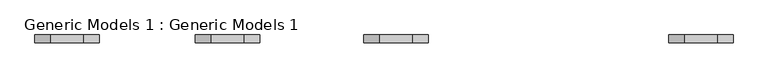
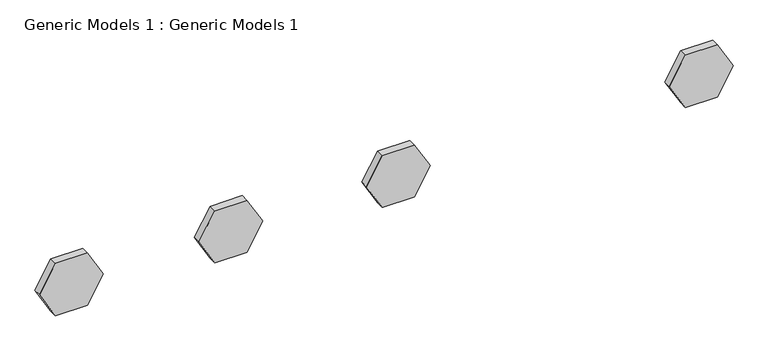
"""IFC4 building model written with IfcOpenShell, lengths in millimetres: proxy geometry, Generic Models 1 : Generic Models 1."""

from ifc_helpers import new_model, si_unit, frame, origin, place, context, project, spatial, polyline, outline, extrude, source, transform, mapped, element, save


def generic_models_1_generic_models_1_46fdab30(model_context):
    return source(origin(), model_context, "Body", "SweptSolid", [
        extrude(outline(polyline([(1354.8156911, 5498.4896844), (1354.8156911, 4888.8896844), (826.8866049, 4584.0896844), (298.9575188, 4888.8896844), (298.9575188, 5498.4896844), (826.8866049, 5803.2896844), (1354.8156911, 5498.4896844)])), frame((0.0, -9884.41366, 0.0), z_axis=(0.0, 1.0, 0.0), x_axis=(0.0, 0.0, 1.0)), (0.0, 0.0, 1.0), 152.4),
        extrude(outline(polyline([(1354.8156911, -292.7103156), (1354.8156911, -902.3103156), (826.8866049, -1207.1103156), (298.9575188, -902.3103156), (298.9575188, -292.7103156), (826.8866049, 12.0896844), (1354.8156911, -292.7103156)])), frame((0.0, -9884.41366, 0.0), z_axis=(0.0, 1.0, 0.0), x_axis=(0.0, 0.0, 1.0)), (0.0, 0.0, 1.0), 152.4),
        extrude(outline(polyline([(1354.8156911, -3492.110926), (1354.8156911, -4101.710926), (826.8866049, -4406.510926), (298.9575188, -4101.710926), (298.9575188, -3492.110926), (826.8866049, -3187.310926), (1354.8156911, -3492.110926)])), frame((0.0, -9884.41366, 0.0), z_axis=(0.0, 1.0, 0.0), x_axis=(0.0, 0.0, 1.0)), (0.0, 0.0, 1.0), 152.4),
        extrude(outline(polyline([(1354.8156911, -6540.110926), (1354.8156911, -7149.710926), (826.8866049, -7454.510926), (298.9575188, -7149.710926), (298.9575188, -6540.110926), (826.8866049, -6235.310926), (1354.8156911, -6540.110926)])), frame((0.0, -9884.41366, 0.0), z_axis=(0.0, 1.0, 0.0), x_axis=(0.0, 0.0, 1.0)), (0.0, 0.0, 1.0), 152.4),
    ])


if __name__ == "__main__":
    model = new_model("IFC4")
    model_context = context("Model", 3, world=origin())
    ifc_project = project(units=[si_unit("LENGTHUNIT", "METRE", prefix="MILLI")], contexts=[model_context])
    site = spatial("IfcSite", under=ifc_project)
    building = spatial("IfcBuilding", under=site)
    placement = place(None, origin())
    generic_models_1_generic_models_1_shape = generic_models_1_generic_models_1_46fdab30(model_context)
    element("IfcBuildingElementProxy", 1, Name="Generic Models 1 : Generic Models 1", ObjectType="Generic Models 1 : Generic Models 1", at=placement, inside=building, context=model_context, shape_type="MappedRepresentation", body=[
        mapped(generic_models_1_generic_models_1_shape, transform((0.0, 0.0, 0.0), x_axis=(1.0, 0.0, 0.0), y_axis=(0.0, 1.0, 0.0), z_axis=(0.0, 0.0, 1.0))),
    ])
    save(model, "model.ifc")

# Revit data of these elements
# Element 1 (IfcBuildingElementProxy, "Generic Models 1 : Generic Models 1")
#   Materials on its faces: "Parking Stripe"
# Materials
#   "Parking Stripe": class "Paint", colour RGB 250 250 91, transparency 0, Cost = 0
